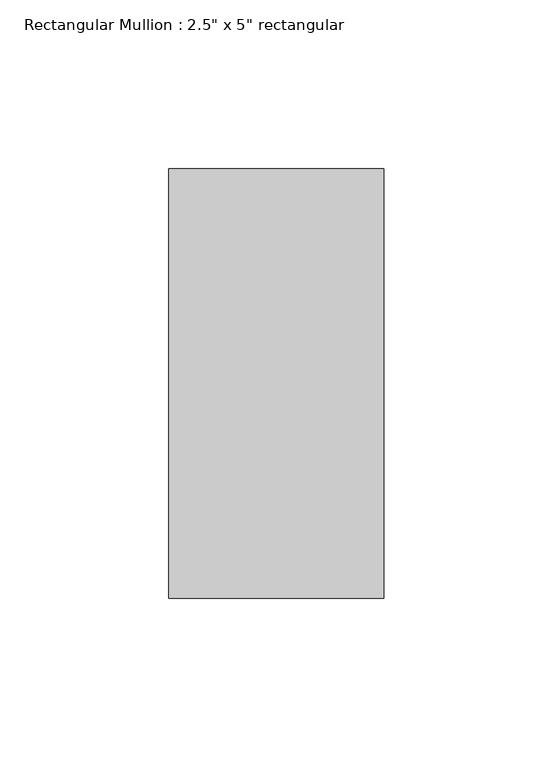
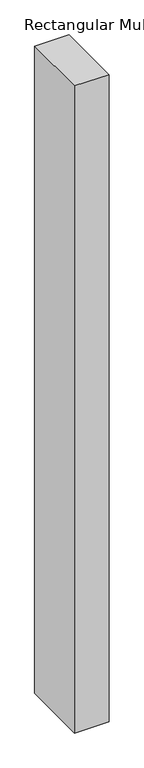
"""IFC4 building model written with IfcOpenShell, lengths in millimetres: member geometry."""

from ifc_helpers import new_model, si_unit, frame, origin, place, context, project, spatial, polyline, outline, extrude, source, transform, mapped, element, save


def member_bcb6a316(model_context):
    return source(origin(), model_context, "Body", "SweptSolid", [
        extrude(outline(polyline([(0.0, 63.5), (0.0, -63.5), (-63.5, -63.5), (-63.5, 63.5), (0.0, 63.5)])), frame((0.0, 0.0, -1257.3), z_axis=(0.0, 0.0, 1.0), x_axis=(1.0, 0.0, 0.0)), (0.0, 0.0, 1.0), 1257.3),
    ])


if __name__ == "__main__":
    model = new_model("IFC4")
    model_context = context("Model", 3, world=origin())
    ifc_project = project(units=[si_unit("LENGTHUNIT", "METRE", prefix="MILLI")], contexts=[model_context])
    site = spatial("IfcSite", under=ifc_project)
    building = spatial("IfcBuilding", under=site)
    placement = place(None, origin())
    member_shape = member_bcb6a316(model_context)
    element("IfcMember", 1, ObjectType="Rectangular Mullion : 2.5\" x 5\" rectangular", at=placement, inside=building, context=model_context, shape_type="MappedRepresentation", body=[
        mapped(member_shape, transform((0.0, 0.0, 0.0), x_axis=(1.0, 0.0, 0.0), y_axis=(0.0, 1.0, 0.0), z_axis=(0.0, 0.0, 1.0))),
    ])
    save(model, "model.ifc")

# Revit data of these elements
# Type "Rectangular Mullion : 2.5\" x 5\" rectangular"
#   built-in parameter 1007304 = 0.416667 (stored number, unit not read)
#   built-in parameter 1007301 = 0.104167 (stored number, unit not read)
#   built-in parameter 1007300 = 0.104167 (stored number, unit not read)
# Element 1 (IfcMember, "Rectangular Mullion : 2.5\" x 5\" rectangular")
#   Materials on its faces: "Aluminum"
# Materials
#   "Aluminum": class "Metal", colour RGB 247 247 247, transparency 0, Description = "Aluminum 6061", Cost = 0
